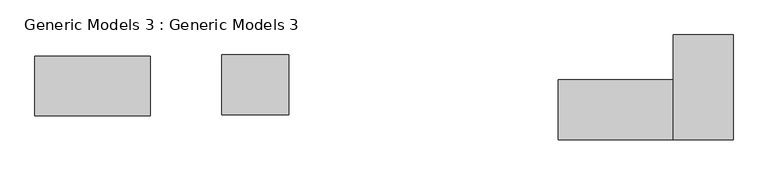
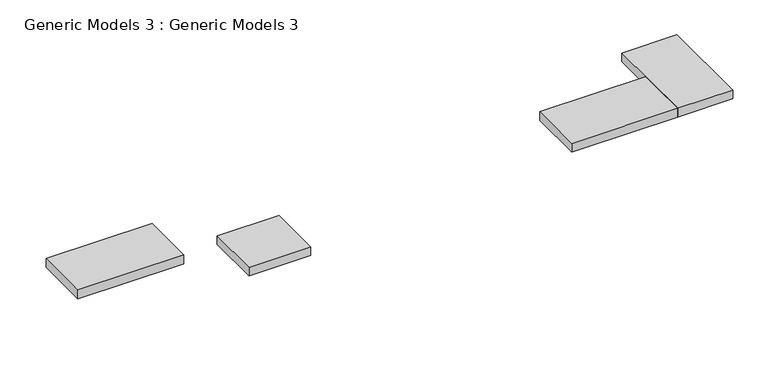
"""IFC4 building model written with IfcOpenShell, lengths in millimetres: proxy geometry, Generic Models 3 : Generic Models 3."""

from ifc_helpers import new_model, si_unit, frame, origin, place, context, project, spatial, polyline, outline, extrude, source, transform, mapped, element, save


def generic_models_3_generic_models_3_1965cac1(model_context):
    return source(origin(), model_context, "Body", "SweptSolid", [
        extrude(outline(polyline([(2800.35, -40314.6645004), (2952.75, -40314.6645004), (2952.75, -42073.6145004), (2800.35, -42073.6145004), (2800.35, -40467.0645004), (2800.35, -40314.6645004)])), frame((0.0, 5090.4756148, 0.0), z_axis=(0.0, 1.0, 0.0), x_axis=(0.0, 0.0, 1.0)), (0.0, 0.0, 1.0), 914.4),
        extrude(outline(polyline([(2190.75, -39222.4645004), (2190.75, -39070.0645004), (2190.75, -38346.1645004), (2190.75, -38193.7645004), (2343.15, -38193.7645004), (2343.15, -39222.4645004), (2190.75, -39222.4645004)])), frame((0.0, 5109.5256148, 0.0), z_axis=(0.0, 1.0, 0.0), x_axis=(0.0, 0.0, 1.0)), (0.0, 0.0, 1.0), 914.4),
        extrude(outline(polyline([(-31405.6145004, 6328.7256148), (-31405.6145004, 4728.4472085), (-32320.0145004, 4728.4472085), (-32320.0145004, 6328.7256148), (-31405.6145004, 6328.7256148)])), frame((0.0, 0.0, 2800.35), z_axis=(0.0, 0.0, 1.0), x_axis=(1.0, 0.0, 0.0)), (0.0, 0.0, 1.0), 152.4),
        extrude(outline(polyline([(2800.35, -34078.9645004), (2800.35, -33926.5645004), (2800.35, -32320.0145004), (2952.75, -32320.0145004), (2952.75, -34078.9645004), (2800.35, -34078.9645004)])), frame((0.0, 4728.4472085, 0.0), z_axis=(0.0, 1.0, 0.0), x_axis=(0.0, 0.0, 1.0)), (0.0, 0.0, 1.0), 914.4),
    ])


if __name__ == "__main__":
    model = new_model("IFC4")
    model_context = context("Model", 3, world=origin())
    ifc_project = project(units=[si_unit("LENGTHUNIT", "METRE", prefix="MILLI")], contexts=[model_context])
    site = spatial("IfcSite", under=ifc_project)
    building = spatial("IfcBuilding", under=site)
    placement = place(None, origin())
    generic_models_3_generic_models_3_shape = generic_models_3_generic_models_3_1965cac1(model_context)
    element("IfcBuildingElementProxy", 1, Name="Generic Models 3 : Generic Models 3", ObjectType="Generic Models 3 : Generic Models 3", at=placement, inside=building, context=model_context, shape_type="MappedRepresentation", body=[
        mapped(generic_models_3_generic_models_3_shape, transform((0.0, 0.0, 0.0), x_axis=(1.0, 0.0, 0.0), y_axis=(0.0, 1.0, 0.0), z_axis=(0.0, 0.0, 1.0))),
    ])
    save(model, "model.ifc")
